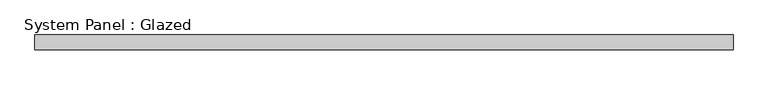
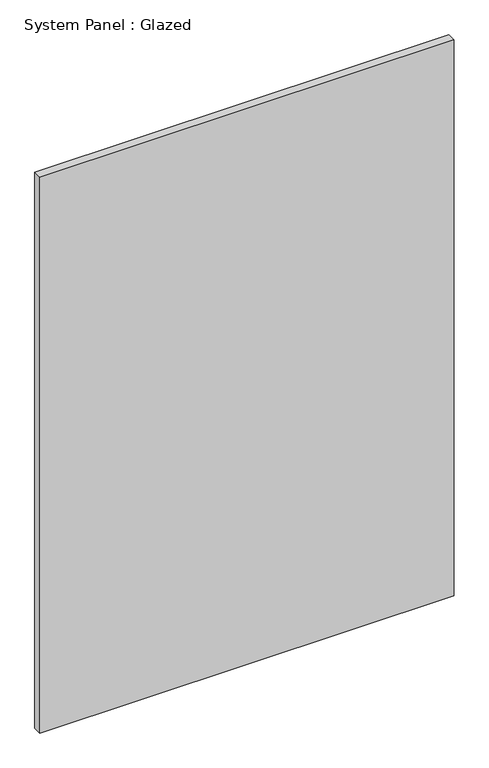
"""IFC4 building model written with IfcOpenShell, lengths in millimetres: plate geometry, System Panel : Glazed."""

from ifc_helpers import new_model, si_unit, origin, origin_with_axes, place, context, project, spatial, polyline, outline, extrude, source, transform, mapped, element, save


def system_panel_glazed_8590af86(model_context):
    return source(origin(), model_context, "Body", "SweptSolid", [
        extrude(outline(polyline([(600.075, 19.05), (-600.075, 19.05), (-600.075, 44.45), (600.075, 44.45), (600.075, 19.05)])), origin_with_axes(), (0.0, 0.0, 1.0), 1701.8),
    ])


if __name__ == "__main__":
    model = new_model("IFC4")
    model_context = context("Model", 3, world=origin())
    ifc_project = project(units=[si_unit("LENGTHUNIT", "METRE", prefix="MILLI")], contexts=[model_context])
    site = spatial("IfcSite", under=ifc_project)
    building = spatial("IfcBuilding", under=site)
    placement = place(None, origin())
    system_panel_glazed_shape = system_panel_glazed_8590af86(model_context)
    element("IfcPlate", 1, ObjectType="System Panel : Glazed", at=placement, inside=building, context=model_context, shape_type="MappedRepresentation", body=[
        mapped(system_panel_glazed_shape, transform((0.0, 0.0, 0.0), x_axis=(1.0, 0.0, 0.0), y_axis=(0.0, 1.0, 0.0), z_axis=(0.0, 0.0, 1.0))),
    ])
    save(model, "model.ifc")

# Revit data of these elements
# Type "System Panel : Glazed"
#   Construction Type Id = "GSP4R"
#   Analytic Construction = "1/8 in Pilkington single glazing"
#   Visual Light Transmittance = 0.9
#   Solar Heat Gain Coefficient = 0.86
#   Heat Transfer Coefficient (U) = 1.18115 BTU/(h·ft²·°F)
# Element 1 (IfcPlate, "System Panel : Glazed")
#   Materials on its faces: "Glass"
# Materials
#   "Glass": class "Glass", colour RGB 0 128 192, transparency 0.75, Description = "Soda Lime Glass", Cost = 0
